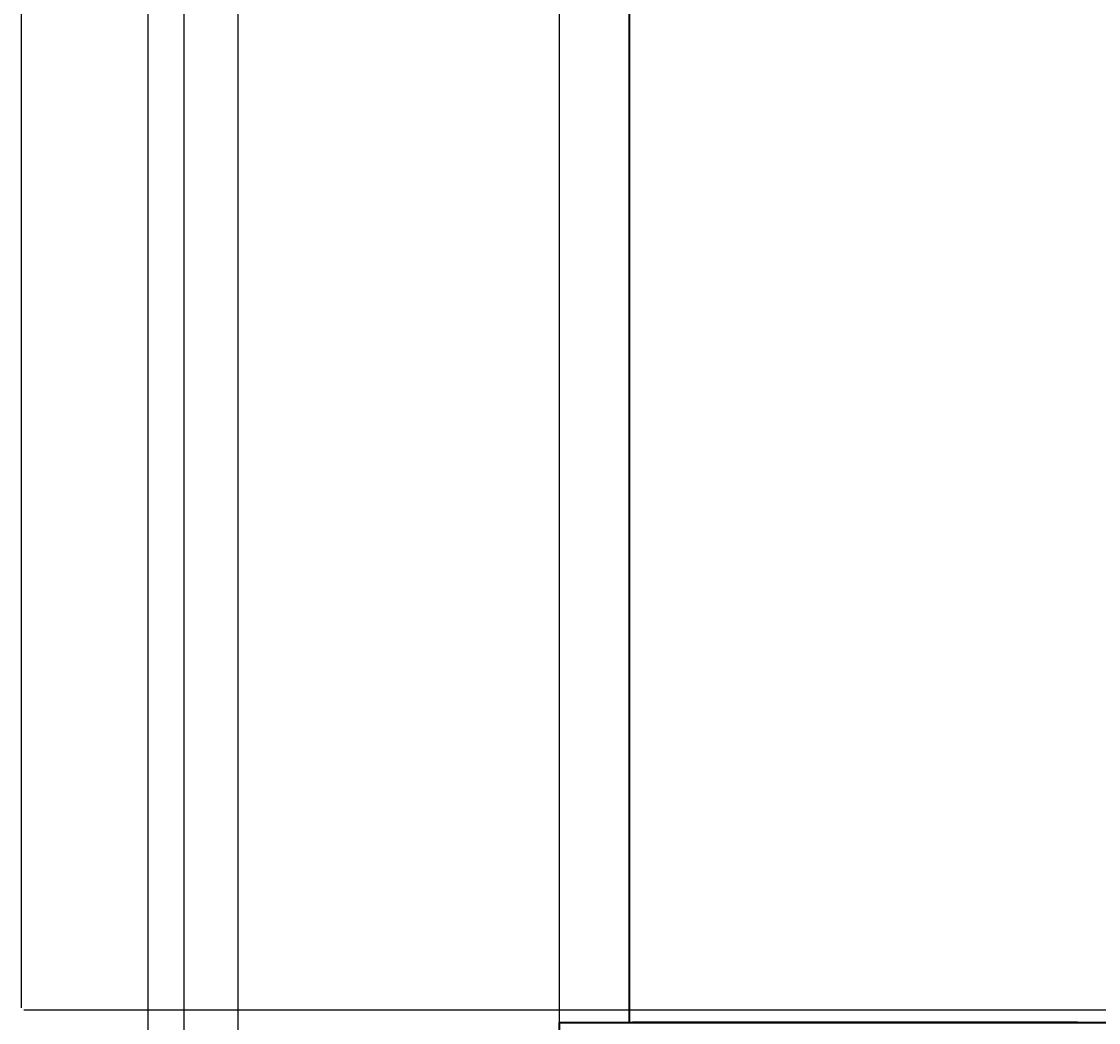
# Model space of a CAD drawing. Units: inches. Extents: x -6 to 289, y -8 to 323.
# Tile 39 of 107: x 230 to 260, y 68 to 96. Entities that reach past the tile are written whole.
import ezdxf

# ---------------------------------------------------------------- set-up
doc = ezdxf.new("R2010")
doc.units = ezdxf.units.IN
doc.header["$MEASUREMENT"] = 0
doc.layers.add('A-ANNO-DIMS', color=2, linetype='Continuous', lineweight=18)
doc.layers.add('A-ELEV', color=7, linetype='Continuous', lineweight=35)
doc.styles.get("Standard").update_dxf_attribs({"font": 'arial.ttf'})
doc.dimstyles.get("Standard").update_dxf_attribs({"dimtxt": 0.18, "dimasz": 0.18, "dimexe": 0.18, "dimexo": 0.0625, "dimgap": 0.09, "dimtad": 0, "dimtih": 1, "dimtoh": 1, "dimdec": 4, "dimzin": 0, "dimdsep": 46, "dimtxsty": 'Standard', "dimcen": 0.09, "dimadec": 0, "dimazin": 0, "dimtfac": 1, "dimtdec": 4, "dimtofl": 0, "dimtmove": 0, "dimatfit": 3, "dimfxl": 1, "dimtolj": 1, "dimtzin": 0, "dimarcsym": 0})

# ---------------------------------------------------------------- blocks, each defined once
blk = doc.blocks.new('*D15')
at = {"layer": 'A-ANNO-DIMS', "color": 0, "lineweight": -2, "transparency": 16777216}
for p, q in [((247.164, 162.411), (247.164, 322.969)), ((247.344, 322.789), (258.944, 322.789)), ((270.984, 322.789), (259.384, 322.789)), ((271.164, 7.351), (271.164, 322.969))]:
    blk.add_line(p, q, dxfattribs=at)
at = {"layer": 'A-ANNO-DIMS', "color": 0, "transparency": 16777216}
for points in [[(247.344, 322.819), (247.344, 322.759), (247.164, 322.789)], [(270.984, 322.819), (270.984, 322.759), (271.164, 322.789)]]:
    blk.add_solid(points, dxfattribs=at)
at = {"layer": 'Defpoints', "color": 0, "transparency": 16777216}
for p in [(271.164, 322.789), (247.164, 162.348), (271.164, 7.289)]:
    blk.add_point(p, dxfattribs=at)
at = {"layer": 'A-ANNO-DIMS', "color": 0, "transparency": 16777216, "insert": (259.164, 322.789), "char_height": 0.18, "attachment_point": 5}
blk.add_mtext('\\A1;24', dxfattribs=at)
blk = doc.blocks.new('*D23')
at = {"layer": 'A-ANNO-DIMS', "color": 0, "lineweight": -2, "transparency": 16777216}
for p, q in [((259.226, 127.289), (288.653, 127.289)), ((288.473, 127.109), (288.473, 67.471)), ((288.473, 7.469), (288.473, 67.107)), ((271.226, 7.289), (288.653, 7.289))]:
    blk.add_line(p, q, dxfattribs=at)
at = {"layer": 'A-ANNO-DIMS', "color": 0, "transparency": 16777216}
for points in [[(288.443, 127.109), (288.503, 127.109), (288.473, 127.289)], [(288.443, 7.469), (288.503, 7.469), (288.473, 7.289)]]:
    blk.add_solid(points, dxfattribs=at)
at = {"layer": 'Defpoints', "color": 0, "transparency": 16777216}
for p in [(259.164, 127.289), (288.473, 127.289), (271.164, 7.289)]:
    blk.add_point(p, dxfattribs=at)
at = {"layer": 'A-ANNO-DIMS', "color": 0, "transparency": 16777216, "insert": (288.473, 67.289), "char_height": 0.18, "attachment_point": 5}
blk.add_mtext('\\A1;120', dxfattribs=at)
blk = doc.blocks.new('*D44')
at = {"layer": 'A-ANNO-DIMS', "color": 0, "lineweight": -2, "transparency": 16777216}
for p, q in [((212.292, 224.326), (212.292, -8.391)), ((233.792, 224.326), (233.792, -8.391)), ((212.472, -8.211), (222.716, -8.211)), ((233.612, -8.211), (223.368, -8.211))]:
    blk.add_line(p, q, dxfattribs=at)
at = {"layer": 'A-ANNO-DIMS', "color": 0, "transparency": 16777216}
for points in [[(212.472, -8.181), (212.472, -8.241), (212.292, -8.211)], [(233.612, -8.181), (233.612, -8.241), (233.792, -8.211)]]:
    blk.add_solid(points, dxfattribs=at)
at = {"layer": 'Defpoints', "color": 0, "transparency": 16777216}
for p in [(212.292, 224.389), (233.792, 224.389), (233.792, -8.211)]:
    blk.add_point(p, dxfattribs=at)
at = {"layer": 'A-ANNO-DIMS', "color": 0, "transparency": 16777216, "insert": (223.042, -8.211), "char_height": 0.18, "attachment_point": 5}
blk.add_mtext('\\A1;21.5', dxfattribs=at)
blk = doc.blocks.new('*D45')
at = {"layer": 'A-ANNO-DIMS', "color": 0, "lineweight": -2, "transparency": 16777216}
for p, q in [((234.792, 225.326), (234.792, -8.391)), ((233.792, 224.326), (233.792, -8.391)), ((233.972, -8.211), (234.169, -8.211)), ((234.612, -8.211), (234.415, -8.211))]:
    blk.add_line(p, q, dxfattribs=at)
at = {"layer": 'A-ANNO-DIMS', "color": 0, "transparency": 16777216}
for points in [[(233.972, -8.181), (233.972, -8.241), (233.792, -8.211)], [(234.612, -8.181), (234.612, -8.241), (234.792, -8.211)]]:
    blk.add_solid(points, dxfattribs=at)
at = {"layer": 'Defpoints', "color": 0, "transparency": 16777216}
for p in [(234.792, 225.389), (233.792, 224.389), (234.792, -8.211)]:
    blk.add_point(p, dxfattribs=at)
at = {"layer": 'A-ANNO-DIMS', "color": 0, "transparency": 16777216, "insert": (234.292, -8.211), "char_height": 0.18, "attachment_point": 5}
blk.add_mtext('\\A1;1', dxfattribs=at)
blk = doc.blocks.new('*D46')
at = {"layer": 'A-ANNO-DIMS', "color": 0, "lineweight": -2, "transparency": 16777216}
for p, q in [((236.292, 226.826), (236.292, -8.391)), ((234.792, 225.326), (234.792, -8.391)), ((234.972, -8.211), (235.296, -8.211)), ((236.112, -8.211), (235.788, -8.211))]:
    blk.add_line(p, q, dxfattribs=at)
at = {"layer": 'A-ANNO-DIMS', "color": 0, "transparency": 16777216}
for points in [[(234.972, -8.181), (234.972, -8.241), (234.792, -8.211)], [(236.112, -8.181), (236.112, -8.241), (236.292, -8.211)]]:
    blk.add_solid(points, dxfattribs=at)
at = {"layer": 'Defpoints', "color": 0, "transparency": 16777216}
for p in [(236.292, 226.889), (234.792, 225.389), (236.292, -8.211)]:
    blk.add_point(p, dxfattribs=at)
at = {"layer": 'A-ANNO-DIMS', "color": 0, "transparency": 16777216, "insert": (235.542, -8.211), "char_height": 0.18, "attachment_point": 5}
blk.add_mtext('\\A1;1.5', dxfattribs=at)
blk = doc.blocks.new('*D81')
at = {"layer": 'A-ANNO-DIMS', "color": 0, "lineweight": -2, "transparency": 16777216}
for p, q in [((230.292, 68.842), (230.292, 322.969)), ((230.472, 322.789), (237.298, 322.789)), ((245.035, 322.789), (238.208, 322.789)), ((245.215, 66.286), (245.215, 322.969))]:
    blk.add_line(p, q, dxfattribs=at)
at = {"layer": 'A-ANNO-DIMS', "color": 0, "transparency": 16777216}
for points in [[(230.472, 322.819), (230.472, 322.759), (230.292, 322.789)], [(245.035, 322.819), (245.035, 322.759), (245.215, 322.789)]]:
    blk.add_solid(points, dxfattribs=at)
at = {"layer": 'Defpoints', "color": 0, "transparency": 16777216}
for p in [(245.215, 322.789), (230.292, 68.779), (245.215, 66.224)]:
    blk.add_point(p, dxfattribs=at)
at = {"layer": 'A-ANNO-DIMS', "color": 0, "transparency": 16777216, "insert": (237.753, 322.789), "char_height": 0.18, "attachment_point": 5}
blk.add_mtext('\\A1;14.923', dxfattribs=at)
blk = doc.blocks.new('*D82')
at = {"layer": 'A-ANNO-DIMS', "color": 0, "lineweight": -2, "transparency": 16777216}
for p, q in [((245.215, 66.286), (245.215, 322.969)), ((245.395, 322.789), (258.699, 322.789)), ((272.793, 322.789), (259.489, 322.789)), ((272.973, 66.286), (272.973, 322.969))]:
    blk.add_line(p, q, dxfattribs=at)
at = {"layer": 'A-ANNO-DIMS', "color": 0, "transparency": 16777216}
for points in [[(245.395, 322.819), (245.395, 322.759), (245.215, 322.789)], [(272.793, 322.819), (272.793, 322.759), (272.973, 322.789)]]:
    blk.add_solid(points, dxfattribs=at)
at = {"layer": 'Defpoints', "color": 0, "transparency": 16777216}
for p in [(272.973, 322.789), (245.215, 66.224), (272.973, 66.224)]:
    blk.add_point(p, dxfattribs=at)
at = {"layer": 'A-ANNO-DIMS', "color": 0, "transparency": 16777216, "insert": (259.094, 322.789), "char_height": 0.18, "attachment_point": 5}
blk.add_mtext('\\A1;27.76', dxfattribs=at)
blk = doc.blocks.new('*D90')
at = {"layer": 'A-ANNO-DIMS', "color": 0, "lineweight": -2, "transparency": 16777216}
for p, q in [((230.354, 68.779), (288.653, 68.779)), ((288.473, 68.599), (288.473, 60.114)), ((288.473, 51.265), (288.473, 59.75)), ((247.303, 51.085), (288.653, 51.085))]:
    blk.add_line(p, q, dxfattribs=at)
at = {"layer": 'A-ANNO-DIMS', "color": 0, "transparency": 16777216}
for points in [[(288.443, 68.599), (288.503, 68.599), (288.473, 68.779)], [(288.443, 51.265), (288.503, 51.265), (288.473, 51.085)]]:
    blk.add_solid(points, dxfattribs=at)
at = {"layer": 'Defpoints', "color": 0, "transparency": 16777216}
for p in [(230.292, 68.779), (288.473, 68.779), (247.241, 51.085)]:
    blk.add_point(p, dxfattribs=at)
at = {"layer": 'A-ANNO-DIMS', "color": 0, "transparency": 16777216, "insert": (288.473, 59.932), "char_height": 0.18, "attachment_point": 5}
blk.add_mtext('\\A1;17.694', dxfattribs=at)
blk = doc.blocks.new('*D91')
at = {"layer": 'A-ANNO-DIMS', "color": 0, "lineweight": -2, "transparency": 16777216}
for p, q in [((230.354, 116.779), (288.653, 116.779)), ((288.473, 116.599), (288.473, 92.961)), ((288.473, 68.959), (288.473, 92.598)), ((230.354, 68.779), (288.653, 68.779))]:
    blk.add_line(p, q, dxfattribs=at)
at = {"layer": 'A-ANNO-DIMS', "color": 0, "transparency": 16777216}
for points in [[(288.443, 116.599), (288.503, 116.599), (288.473, 116.779)], [(288.443, 68.959), (288.503, 68.959), (288.473, 68.779)]]:
    blk.add_solid(points, dxfattribs=at)
at = {"layer": 'Defpoints', "color": 0, "transparency": 16777216}
for p in [(230.292, 116.779), (288.473, 116.779), (230.292, 68.779)]:
    blk.add_point(p, dxfattribs=at)
at = {"layer": 'A-ANNO-DIMS', "color": 0, "transparency": 16777216, "insert": (288.473, 92.779), "char_height": 0.18, "attachment_point": 5}
blk.add_mtext('\\A1;48', dxfattribs=at)

msp = doc.modelspace()

# ---------------------------------------------------------------- linework, layer by layer
at = {"layer": 'A-ELEV'}
msp.add_line((247.1638, 68.4323), (247.1638, 127.2888), dxfattribs=at)
msp.add_lwpolyline([(245.2146, 68.4323), (272.9733, 68.4323), (272.9733, 66.2238), (245.2146, 66.2238)], close=True, dxfattribs=at)
msp.add_lwpolyline([(259.5885, 68.4323), (247.2408, 68.4323)], dxfattribs=at)

# ---------------------------------------------------------------- dimensions: what is measured, and where the dimension line sits
at = {"layer": 'A-ANNO-DIMS'}
for base, p1, p2, override, picture, middle in [((245.2146, 322.7888), (230.2918, 68.7795), (245.2146, 66.2238), {"dimdec": 3, "dimlfac": 1, "dimrnd": 0, "dimzin": 0, "dimdsep": 46, "dimlunit": 2}, '*D81', (237.7532, 322.7888)), ((272.9733, 322.7888), (245.2146, 66.2238), (272.9733, 66.2238), {"dimdec": 2, "dimlfac": 1, "dimrnd": 0, "dimzin": 0, "dimdsep": 46, "dimlunit": 2}, '*D82', (259.0939, 322.7888)), ((271.1638, 322.7888), (247.1638, 162.3484), (271.1638, 7.2888), {"dimdec": 0, "dimlfac": 1, "dimrnd": 0, "dimzin": 0, "dimdsep": 46, "dimlunit": 2}, '*D15', (259.1638, 322.7888)), ((236.2918, -8.2112), (234.7918, 225.3887), (236.2918, 226.8887), {"dimdec": 1, "dimlfac": 1, "dimrnd": 0, "dimzin": 0, "dimdsep": 46, "dimlunit": 2}, '*D46', (235.5418, -8.2112)), ((234.7918, -8.2112), (233.7918, 224.3887), (234.7918, 225.3887), {"dimdec": 0, "dimlfac": 1, "dimrnd": 0, "dimzin": 0, "dimdsep": 46, "dimlunit": 2}, '*D45', (234.2918, -8.2112)), ((233.7918, -8.2112), (212.2918, 224.3887), (233.7918, 224.3887), {"dimdec": 1, "dimlfac": 1, "dimrnd": 0, "dimzin": 0, "dimdsep": 46, "dimlunit": 2}, '*D44', (223.0418, -8.2112))]:
    dim = msp.add_linear_dim(base=base, p1=p1, p2=p2, dimstyle='Standard', override=override, dxfattribs=at)
    dim.commit()
    dim.dimension.update_dxf_attribs({"geometry": picture, "text_midpoint": middle})
for base, p1, p2, override, picture, middle in [((288.4733, 127.2888), (271.1638, 7.2888), (259.1638, 127.2888), {"dimdec": 0, "dimlfac": 1, "dimrnd": 0, "dimzin": 0, "dimdsep": 46, "dimlunit": 2}, '*D23', (288.4733, 67.2888)), ((288.4733, 116.7795), (230.2918, 68.7795), (230.2918, 116.7795), {"dimdec": 0, "dimlfac": 1, "dimrnd": 0, "dimzin": 0, "dimdsep": 46, "dimlunit": 2}, '*D91', (288.4733, 92.7795)), ((288.4733, 68.7795), (247.2408, 51.0851), (230.2918, 68.7795), {"dimdec": 3, "dimlfac": 1, "dimrnd": 0, "dimzin": 0, "dimdsep": 46, "dimlunit": 2}, '*D90', (288.4733, 59.9323))]:
    dim = msp.add_linear_dim(base=base, p1=p1, p2=p2, angle=90, dimstyle='Standard', override=override, dxfattribs=at)
    dim.commit()
    dim.dimension.update_dxf_attribs({"geometry": picture, "text_midpoint": middle})

doc.saveas('drawing.dxf')
